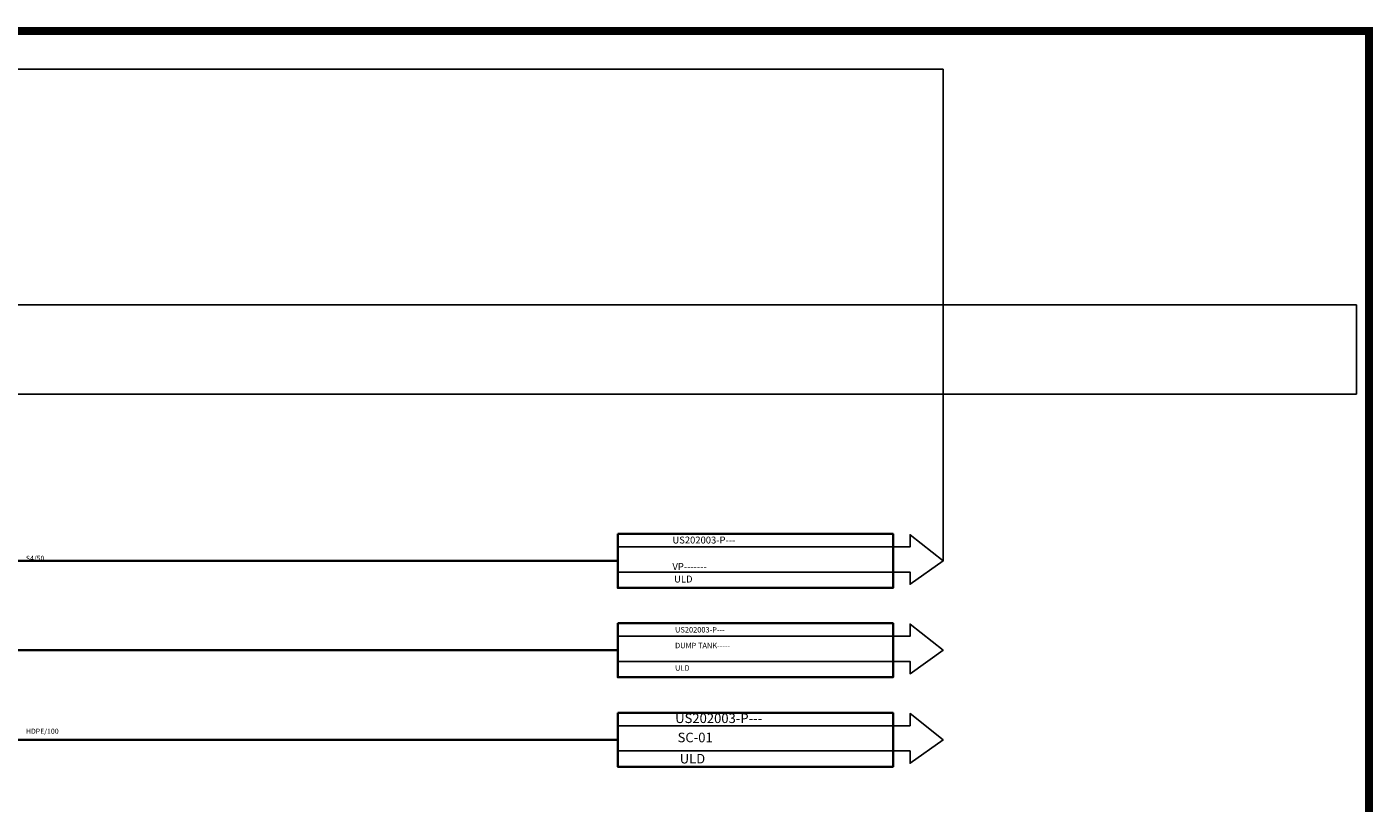
# Model space of a CAD drawing. Units: millimetres. Extents: x 353872 to 441597, y 126154 to 187356.
# Tile 28 of 28: x 415084 to 440911, y 172470 to 187356. Entities that reach past the tile are written whole.
import ezdxf

# ---------------------------------------------------------------- set-up
doc = ezdxf.new("R2010")
doc.units = ezdxf.units.MM
for name, color, linetype, lineweight in [('A-ANNO-DIMS', 2, 'Continuous', 18), ('P-ANNO-TEXT', 7, 'Continuous', 25), ('P-ANNO-TTLB', 7, 'Continuous', 25), ('P-EQPM', 5, 'Continuous', 35), ('P-PIPE', 3, 'Continuous', 35)]:
    doc.layers.add(name, color=color, linetype=linetype, lineweight=lineweight)
doc.styles.get("Standard").update_dxf_attribs({"font": 'arial.ttf'})
doc.dimstyles.get("Standard").update_dxf_attribs({"dimtxt": 0.18, "dimasz": 0.18, "dimexe": 0.18, "dimexo": 0.0625, "dimgap": 0.09, "dimtad": 0, "dimtih": 1, "dimtoh": 1, "dimdec": 4, "dimzin": 0, "dimdsep": 46, "dimtxsty": 'Standard', "dimcen": 0.09, "dimadec": 0, "dimazin": 0, "dimtfac": 1, "dimtdec": 4, "dimtofl": 0, "dimtmove": 0, "dimatfit": 3, "dimfxl": 1, "dimtolj": 1, "dimtzin": 0, "dimarcsym": 0})

# ---------------------------------------------------------------- blocks, each defined once
blk = doc.blocks.new('*D24')
at = {"layer": 'A-ANNO-DIMS', "color": 0, "lineweight": -2, "transparency": 16777216}
for p, q in [((360737, 182546), (360737, 186546)), ((360737, 186546), (396698, 186546)), ((432661, 186546), (396699, 186546)), ((432661, 177114), (432661, 186546))]:
    blk.add_line(p, q, dxfattribs=at)
at = {"layer": 'A-ANNO-DIMS', "color": 0, "transparency": 16777216}
for points in [[(360737, 186546), (360737, 186546), (360737, 186546)], [(432661, 186546), (432661, 186546), (432661, 186546)]]:
    blk.add_solid(points, dxfattribs=at)
at = {"layer": 'Defpoints', "color": 0, "transparency": 16777216}
for p in [(432661, 186546), (360737, 182546), (432661, 177114)]:
    blk.add_point(p, dxfattribs=at)
at = {"layer": 'A-ANNO-DIMS', "color": 0, "transparency": 16777216, "insert": (396699, 186546), "char_height": 0.18, "attachment_point": 5}
blk.add_mtext('\\A1;71924', dxfattribs=at)
blk = doc.blocks.new('*D28')
at = {"layer": 'A-ANNO-DIMS', "color": 0, "lineweight": -2, "transparency": 16777216}
for p, q in [((366977, 182028), (440591, 182028)), ((440591, 182028), (440591, 181171)), ((440591, 180314), (440591, 181171)), ((366977, 180314), (440591, 180314))]:
    blk.add_line(p, q, dxfattribs=at)
at = {"layer": 'A-ANNO-DIMS', "color": 0, "transparency": 16777216}
for points in [[(440591, 182028), (440591, 182028), (440591, 182028)], [(440591, 180314), (440591, 180314), (440591, 180314)]]:
    blk.add_solid(points, dxfattribs=at)
at = {"layer": 'Defpoints', "color": 0, "transparency": 16777216}
for p in [(366977, 182028), (366977, 180314), (440591, 180314)]:
    blk.add_point(p, dxfattribs=at)
at = {"layer": 'A-ANNO-DIMS', "color": 0, "transparency": 16777216, "insert": (440591, 181171), "char_height": 0.18, "attachment_point": 5}
blk.add_mtext('\\A1;1714.5', dxfattribs=at)

msp = doc.modelspace()

# ---------------------------------------------------------------- linework, layer by layer
at = {"layer": 'P-ANNO-TTLB', "const_width": 152.43}
msp.add_lwpolyline([(353948.03, 187280.05), (353948.03, 126916.34), (440835.19, 126916.34), (440835.19, 187280.05)], close=True, dxfattribs=at)
at = {"layer": 'P-ANNO-TTLB'}
for points in [[(426420.76, 176900.33), (432027.57, 176900.33), (432027.57, 176666.35), (432660.97, 177114.41), (432027.57, 177617.46), (432027.57, 177383.48), (426420.76, 177383.48)], [(426420.76, 175185.8), (432027.57, 175185.8), (432027.57, 174951.82), (432660.97, 175399.89), (432027.57, 175902.93), (432027.57, 175668.95), (426420.76, 175668.95)], [(426420.76, 173468.65), (432027.57, 173468.65), (432027.57, 173234.67), (432660.97, 173682.74), (432027.57, 174185.79), (432027.57, 173951.8), (426420.76, 173951.8)]]:
    msp.add_lwpolyline(points, dxfattribs=at)
at = {"layer": 'P-EQPM'}
for points in [[(426420.76, 177632.03), (431701.74, 177632.03), (431701.74, 176596.8), (426420.76, 176596.8)], [(426420.76, 175917.5), (431701.74, 175917.5), (431701.74, 174882.28), (426420.76, 174882.28)], [(426420.76, 174200.35), (431701.74, 174200.35), (431701.74, 173165.13), (426420.76, 173165.13)]]:
    msp.add_lwpolyline(points, close=True, dxfattribs=at)
at = {"layer": 'P-PIPE'}
msp.add_line((426420.76, 173682.74), (403622.45, 173682.74), dxfattribs=at)
msp.add_lwpolyline([(426420.76, 177114.41), (409404.23, 177114.41), (409404.23, 175879.94, -1), (409404.23, 174919.83), (409404.23, 174162.79, -1), (409404.23, 173202.69), (409404.23, 172914.66), (409404.23, 172512.05)], format="xyb", dxfattribs=at)
msp.add_lwpolyline([(393066.71, 149319.73), (393066.71, 175399.89), (426420.76, 175399.89)], dxfattribs=at)

# ---------------------------------------------------------------- texts
at = {"layer": 'P-ANNO-TEXT'}
for s, height, p in [('US202003-P---', 132.6763, (427468.89, 177448.5)), ('S4/50', 98.09, (415064.35, 177114.41)), ('VP-------', 132.676, (427468.89, 176939.65)), ('ULD ', 132.676, (427501.07, 176700.18)), ('US202003-P---', 104.6198, (427519.75, 175741.26)), ('DUMP TANK-----', 104.6198, (427519.75, 175439.02)), ('ULD', 104.62, (427519.75, 175007.52)), ('US202003-P---', 183.3994, (427522.2, 174004.86)), ('HDPE/100', 98.09, (415064.35, 173799.23)), ('SC-01', 183.399, (427568.68, 173636.12)), ('ULD', 183.399, (427609.17, 173229.37))]:
    msp.add_text(s, height=height, dxfattribs=at).set_placement(p)

# ---------------------------------------------------------------- dimensions: what is measured, and where the dimension line sits
at = {"layer": 'A-ANNO-DIMS'}
dim = msp.add_linear_dim(base=(432660.97, 186546.05), p1=(360736.55, 182546.05), p2=(432660.97, 177114.41), dimstyle='Standard', override={"dimdec": 0, "dimlfac": 1, "dimrnd": 0, "dimzin": 0, "dimdsep": 46, "dimlunit": 2}, dxfattribs=at)
dim.commit()
dim.dimension.update_dxf_attribs({"geometry": '*D24', "text_midpoint": (396698.76, 186546.05)})
dim = msp.add_linear_dim(base=(440591, 180313.91), p1=(366976.76, 182028.44), p2=(366976.76, 180313.91), angle=90, dimstyle='Standard', override={"dimdec": 1, "dimlfac": 1, "dimrnd": 0, "dimzin": 0, "dimdsep": 46, "dimlunit": 2}, dxfattribs=at)
dim.commit()
dim.dimension.update_dxf_attribs({"geometry": '*D28', "text_midpoint": (440591, 181171.18)})

doc.saveas('drawing.dxf')
